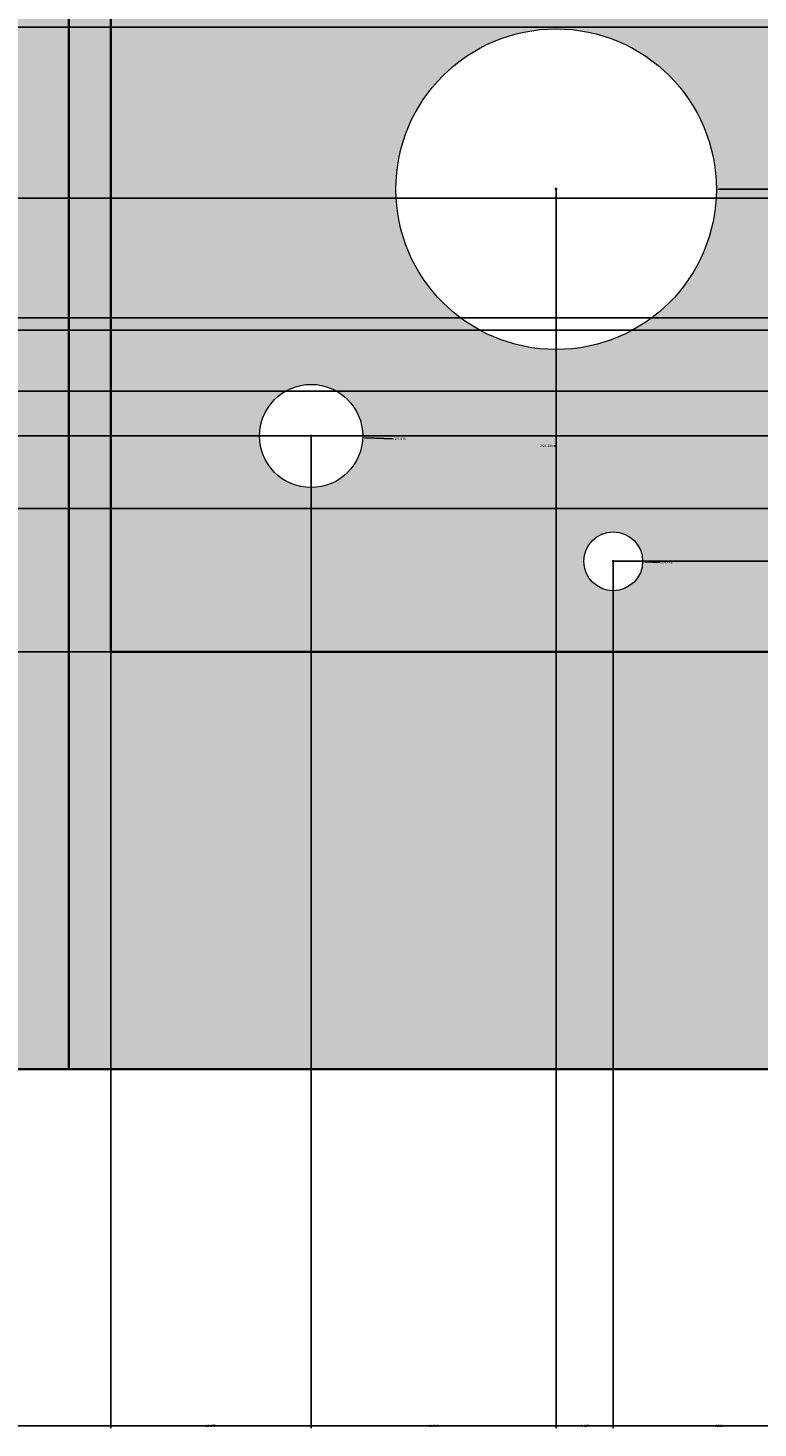
# Model space of a CAD drawing. Units: inches. Extents: x 73 to 607, y 92 to 651.
# Tile 7 of 18: x 448 to 504, y 116 to 222. Entities that reach past the tile are written whole.
import ezdxf

# ---------------------------------------------------------------- set-up
doc = ezdxf.new("R2010")
doc.units = ezdxf.units.IN
doc.header["$MEASUREMENT"] = 0
for name, color, linetype, lineweight in [('A-ANNO-DIMS', 2, 'Continuous', 18), ('A-ELEV', 7, 'Continuous', 35), ('A-ELEV-PANL', 7, 'Continuous', 18), ('A-ELEV-PATT-BKGD', 252, 'Continuous', 13), ('A-ELEV-PATT-SHAD', 8, 'Continuous', 13), ('A-ELEV-PATT-WALL', 254, 'Continuous', 13), ('A-ELEV-PATT-WOOD', 32, 'Continuous', 13)]:
    doc.layers.add(name, color=color, linetype=linetype, lineweight=lineweight)
doc.styles.get("Standard").update_dxf_attribs({"font": 'arial.ttf'})
doc.dimstyles.get("Standard").update_dxf_attribs({"dimtxt": 0.18, "dimasz": 0.18, "dimexe": 0.18, "dimexo": 0.0625, "dimgap": 0.09, "dimtad": 0, "dimtih": 1, "dimtoh": 1, "dimdec": 4, "dimzin": 0, "dimdsep": 46, "dimtxsty": 'Standard', "dimcen": 0.09, "dimadec": 0, "dimazin": 0, "dimtfac": 1, "dimtdec": 4, "dimtofl": 0, "dimtmove": 0, "dimatfit": 3, "dimfxl": 1, "dimtolj": 1, "dimtzin": 0, "dimarcsym": 0})

# ---------------------------------------------------------------- blocks, each defined once
blk = doc.blocks.new('*D4')
at = {"layer": 'A-ANNO-DIMS', "color": 0, "lineweight": -2, "transparency": 16777216}
for p, q in [((100.1, 143.14), (100.1, 116.02)), ((580.1, 143.14), (580.1, 116.02)), ((100.28, 116.2), (339.81, 116.2)), ((579.92, 116.2), (340.39, 116.2))]:
    blk.add_line(p, q, dxfattribs=at)
at = {"layer": 'A-ANNO-DIMS', "color": 0, "transparency": 16777216}
for points in [[(100.28, 116.23), (100.28, 116.17), (100.1, 116.2)], [(579.92, 116.23), (579.92, 116.17), (580.1, 116.2)]]:
    blk.add_solid(points, dxfattribs=at)
at = {"layer": 'Defpoints', "color": 0, "transparency": 16777216}
for p in [(100.1, 143.2), (580.1, 143.2), (580.1, 116.2)]:
    blk.add_point(p, dxfattribs=at)
at = {"layer": 'A-ANNO-DIMS', "color": 0, "transparency": 16777216, "insert": (340.1, 116.2), "char_height": 0.18, "attachment_point": 5}
blk.add_mtext('\\A1;480', dxfattribs=at)
blk = doc.blocks.new('*D15')
at = {"layer": 'A-ANNO-DIMS', "color": 0, "lineweight": -2, "transparency": 16777216}
for p, q in [((454.77, 174.8), (607.28, 174.8)), ((607.1, 174.62), (607.1, 159.19)), ((607.1, 143.38), (607.1, 158.82)), ((580.16, 143.2), (607.28, 143.2))]:
    blk.add_line(p, q, dxfattribs=at)
at = {"layer": 'A-ANNO-DIMS', "color": 0, "transparency": 16777216}
for points in [[(607.07, 174.62), (607.13, 174.62), (607.1, 174.8)], [(607.07, 143.38), (607.13, 143.38), (607.1, 143.2)]]:
    blk.add_solid(points, dxfattribs=at)
at = {"layer": 'Defpoints', "color": 0, "transparency": 16777216}
for p in [(454.7, 174.8), (607.1, 174.8), (580.1, 143.2)]:
    blk.add_point(p, dxfattribs=at)
at = {"layer": 'A-ANNO-DIMS', "color": 0, "transparency": 16777216, "insert": (607.1, 159), "char_height": 0.18, "attachment_point": 5}
blk.add_mtext('\\A1;31.6', dxfattribs=at)
blk = doc.blocks.new('*D16')
at = {"layer": 'A-ANNO-DIMS', "color": 0, "lineweight": -2, "transparency": 16777216}
for p, q in [((431.13, 185.66), (607.28, 185.66)), ((607.1, 185.48), (607.1, 180.41)), ((607.1, 174.98), (607.1, 180.05)), ((454.77, 174.8), (607.28, 174.8))]:
    blk.add_line(p, q, dxfattribs=at)
at = {"layer": 'A-ANNO-DIMS', "color": 0, "transparency": 16777216}
for points in [[(607.07, 185.48), (607.13, 185.48), (607.1, 185.66)], [(607.07, 174.98), (607.13, 174.98), (607.1, 174.8)]]:
    blk.add_solid(points, dxfattribs=at)
at = {"layer": 'Defpoints', "color": 0, "transparency": 16777216}
for p in [(431.07, 185.66), (607.1, 185.66), (454.7, 174.8)]:
    blk.add_point(p, dxfattribs=at)
at = {"layer": 'A-ANNO-DIMS', "color": 0, "transparency": 16777216, "insert": (607.1, 180.23), "char_height": 0.18, "attachment_point": 5}
blk.add_mtext('\\A1;10.86', dxfattribs=at)
blk = doc.blocks.new('*D17')
at = {"layer": 'A-ANNO-DIMS', "color": 0, "lineweight": -2, "transparency": 16777216}
for p, q in [((580.16, 262.3), (607.28, 262.3)), ((607.1, 262.12), (607.1, 224.16)), ((607.1, 185.84), (607.1, 223.8)), ((431.13, 185.66), (607.28, 185.66))]:
    blk.add_line(p, q, dxfattribs=at)
at = {"layer": 'A-ANNO-DIMS', "color": 0, "transparency": 16777216}
for points in [[(607.07, 262.12), (607.13, 262.12), (607.1, 262.3)], [(607.07, 185.84), (607.13, 185.84), (607.1, 185.66)]]:
    blk.add_solid(points, dxfattribs=at)
at = {"layer": 'Defpoints', "color": 0, "transparency": 16777216}
for p in [(580.1, 262.3), (607.1, 262.3), (431.07, 185.66)]:
    blk.add_point(p, dxfattribs=at)
at = {"layer": 'A-ANNO-DIMS', "color": 0, "transparency": 16777216, "insert": (607.1, 223.98), "char_height": 0.18, "attachment_point": 5}
blk.add_mtext('\\A1;76.64', dxfattribs=at)
blk = doc.blocks.new('*D40')
at = {"layer": 'A-ANNO-DIMS', "color": 0, "lineweight": -2, "transparency": 16777216}
for p, q in [((454.64, 256.63), (427.52, 256.63)), ((427.7, 256.45), (427.7, 215.9)), ((427.7, 174.98), (427.7, 215.54)), ((454.64, 174.8), (427.52, 174.8))]:
    blk.add_line(p, q, dxfattribs=at)
at = {"layer": 'A-ANNO-DIMS', "color": 0, "transparency": 16777216}
for points in [[(427.67, 256.45), (427.73, 256.45), (427.7, 256.63)], [(427.67, 174.98), (427.73, 174.98), (427.7, 174.8)]]:
    blk.add_solid(points, dxfattribs=at)
at = {"layer": 'Defpoints', "color": 0, "transparency": 16777216}
for p in [(427.7, 256.63), (454.7, 256.63), (454.7, 174.8)]:
    blk.add_point(p, dxfattribs=at)
at = {"layer": 'A-ANNO-DIMS', "color": 0, "transparency": 16777216, "insert": (427.7, 215.72), "char_height": 0.18, "attachment_point": 5}
blk.add_mtext('\\A1;81.83', dxfattribs=at)
blk = doc.blocks.new('*D62')
at = {"layer": 'A-ANNO-DIMS', "color": 0, "lineweight": -2, "transparency": 16777216}
for p, q in [((488.44, 209.74), (488.44, 209.92)), ((488.35, 209.83), (488.53, 209.83)), ((507.87, 209.83), (500.76, 209.83))]:
    blk.add_line(p, q, dxfattribs=at)
at = {"layer": 'A-ANNO-DIMS', "color": 0, "transparency": 16777216}
blk.add_solid([(500.76, 209.86), (500.76, 209.8), (500.58, 209.83)], dxfattribs=at)
at = {"layer": 'Defpoints', "color": 0, "transparency": 16777216}
for p in [(476.3, 209.83), (500.58, 209.83)]:
    blk.add_point(p, dxfattribs=at)
at = {"layer": 'A-ANNO-DIMS', "color": 0, "transparency": 16777216, "insert": (508.43, 209.83), "char_height": 0.18, "attachment_point": 5}
blk.add_mtext('\\A1;∅24.285', dxfattribs=at)
blk = doc.blocks.new('*D94')
at = {"layer": 'A-ANNO-DIMS', "color": 0, "lineweight": -2, "transparency": 16777216}
for p, q in [((377.02, 209.14), (607.28, 209.14)), ((607.1, 208.96), (607.1, 204.33)), ((607.1, 199.33), (607.1, 203.97)), ((363.32, 199.15), (607.28, 199.15))]:
    blk.add_line(p, q, dxfattribs=at)
at = {"layer": 'A-ANNO-DIMS', "color": 0, "transparency": 16777216}
for points in [[(607.07, 208.96), (607.13, 208.96), (607.1, 209.14)], [(607.07, 199.33), (607.13, 199.33), (607.1, 199.15)]]:
    blk.add_solid(points, dxfattribs=at)
at = {"layer": 'Defpoints', "color": 0, "transparency": 16777216}
for p in [(376.96, 209.14), (363.26, 199.15), (607.1, 199.15)]:
    blk.add_point(p, dxfattribs=at)
at = {"layer": 'A-ANNO-DIMS', "color": 0, "transparency": 16777216, "insert": (607.1, 204.15), "char_height": 0.18, "attachment_point": 5}
blk.add_mtext('\\A1;9.992', dxfattribs=at)
blk = doc.blocks.new('*D95')
at = {"layer": 'A-ANNO-DIMS', "color": 0, "lineweight": -2, "transparency": 16777216}
for p, q in [((363.87, 225.98), (607.28, 225.98)), ((607.1, 225.8), (607.1, 212.75)), ((607.1, 199.33), (607.1, 212.38)), ((363.32, 199.15), (607.28, 199.15))]:
    blk.add_line(p, q, dxfattribs=at)
at = {"layer": 'A-ANNO-DIMS', "color": 0, "transparency": 16777216}
for points in [[(607.07, 225.8), (607.13, 225.8), (607.1, 225.98)], [(607.07, 199.33), (607.13, 199.33), (607.1, 199.15)]]:
    blk.add_solid(points, dxfattribs=at)
at = {"layer": 'Defpoints', "color": 0, "transparency": 16777216}
for p in [(363.81, 225.98), (607.1, 225.98), (363.26, 199.15)]:
    blk.add_point(p, dxfattribs=at)
at = {"layer": 'A-ANNO-DIMS', "color": 0, "transparency": 16777216, "insert": (607.1, 212.57), "char_height": 0.18, "attachment_point": 5}
blk.add_mtext('\\A1;26.83', dxfattribs=at)
blk = doc.blocks.new('*D97')
at = {"layer": 'A-ANNO-DIMS', "color": 0, "lineweight": -2, "transparency": 16777216}
for p, q in [((387.58, 200.08), (607.28, 200.08)), ((607.1, 199.9), (607.1, 197.49)), ((607.1, 194.72), (607.1, 197.12)), ((396.75, 194.54), (607.28, 194.54))]:
    blk.add_line(p, q, dxfattribs=at)
at = {"layer": 'A-ANNO-DIMS', "color": 0, "transparency": 16777216}
for points in [[(607.07, 199.9), (607.13, 199.9), (607.1, 200.08)], [(607.07, 194.72), (607.13, 194.72), (607.1, 194.54)]]:
    blk.add_solid(points, dxfattribs=at)
at = {"layer": 'Defpoints', "color": 0, "transparency": 16777216}
for p in [(387.52, 200.08), (607.1, 200.08), (396.69, 194.54)]:
    blk.add_point(p, dxfattribs=at)
at = {"layer": 'A-ANNO-DIMS', "color": 0, "transparency": 16777216, "insert": (607.1, 197.31), "char_height": 0.18, "attachment_point": 5}
blk.add_mtext('\\A1;5.54', dxfattribs=at)
blk = doc.blocks.new('*D98')
at = {"layer": 'A-ANNO-DIMS', "color": 0, "lineweight": -2, "transparency": 16777216}
for p, q in [((377.02, 209.14), (607.28, 209.14)), ((607.1, 208.96), (607.1, 204.79)), ((607.1, 200.26), (607.1, 204.43)), ((387.58, 200.08), (607.28, 200.08))]:
    blk.add_line(p, q, dxfattribs=at)
at = {"layer": 'A-ANNO-DIMS', "color": 0, "transparency": 16777216}
for points in [[(607.07, 208.96), (607.13, 208.96), (607.1, 209.14)], [(607.07, 200.26), (607.13, 200.26), (607.1, 200.08)]]:
    blk.add_solid(points, dxfattribs=at)
at = {"layer": 'Defpoints', "color": 0, "transparency": 16777216}
for p in [(376.96, 209.14), (607.1, 209.14), (387.52, 200.08)]:
    blk.add_point(p, dxfattribs=at)
at = {"layer": 'A-ANNO-DIMS', "color": 0, "transparency": 16777216, "insert": (607.1, 204.61), "char_height": 0.18, "attachment_point": 5}
blk.add_mtext('\\A1;9.067', dxfattribs=at)
blk = doc.blocks.new('*D99')
at = {"layer": 'A-ANNO-DIMS', "color": 0, "lineweight": -2, "transparency": 16777216}
for p, q in [((373.32, 231.35), (607.28, 231.35)), ((607.1, 231.17), (607.1, 220.43)), ((607.1, 209.32), (607.1, 220.06)), ((377.02, 209.14), (607.28, 209.14))]:
    blk.add_line(p, q, dxfattribs=at)
at = {"layer": 'A-ANNO-DIMS', "color": 0, "transparency": 16777216}
for points in [[(607.07, 231.17), (607.13, 231.17), (607.1, 231.35)], [(607.07, 209.32), (607.13, 209.32), (607.1, 209.14)]]:
    blk.add_solid(points, dxfattribs=at)
at = {"layer": 'Defpoints', "color": 0, "transparency": 16777216}
for p in [(373.26, 231.35), (607.1, 231.35), (376.96, 209.14)]:
    blk.add_point(p, dxfattribs=at)
at = {"layer": 'A-ANNO-DIMS', "color": 0, "transparency": 16777216, "insert": (607.1, 220.25), "char_height": 0.18, "attachment_point": 5}
blk.add_mtext('\\A1;22.205', dxfattribs=at)
blk = doc.blocks.new('*D100')
at = {"layer": 'A-ANNO-DIMS', "color": 0, "lineweight": -2, "transparency": 16777216}
for p, q in [((382.95, 222.1), (607.28, 222.1)), ((607.1, 221.92), (607.1, 211.27)), ((607.1, 200.26), (607.1, 210.9)), ((387.58, 200.08), (607.28, 200.08))]:
    blk.add_line(p, q, dxfattribs=at)
at = {"layer": 'A-ANNO-DIMS', "color": 0, "transparency": 16777216}
for points in [[(607.07, 221.92), (607.13, 221.92), (607.1, 222.1)], [(607.07, 200.26), (607.13, 200.26), (607.1, 200.08)]]:
    blk.add_solid(points, dxfattribs=at)
at = {"layer": 'Defpoints', "color": 0, "transparency": 16777216}
for p in [(382.89, 222.1), (607.1, 222.1), (387.52, 200.08)]:
    blk.add_point(p, dxfattribs=at)
at = {"layer": 'A-ANNO-DIMS', "color": 0, "transparency": 16777216, "insert": (607.1, 211.09), "char_height": 0.18, "attachment_point": 5}
blk.add_mtext('\\A1;22.02', dxfattribs=at)
blk = doc.blocks.new('*D110')
at = {"layer": 'A-ANNO-DIMS', "color": 0, "lineweight": -2, "transparency": 16777216}
for p, q in [((469.88, 191.08), (469.88, 116.02)), ((454.7, 174.74), (454.7, 116.02)), ((454.88, 116.2), (461.84, 116.2)), ((469.7, 116.2), (462.75, 116.2))]:
    blk.add_line(p, q, dxfattribs=at)
at = {"layer": 'A-ANNO-DIMS', "color": 0, "transparency": 16777216}
for points in [[(454.88, 116.23), (454.88, 116.17), (454.7, 116.2)], [(469.7, 116.23), (469.7, 116.17), (469.88, 116.2)]]:
    blk.add_solid(points, dxfattribs=at)
at = {"layer": 'Defpoints', "color": 0, "transparency": 16777216}
for p in [(469.88, 191.14), (454.7, 174.8), (469.88, 116.2)]:
    blk.add_point(p, dxfattribs=at)
at = {"layer": 'A-ANNO-DIMS', "color": 0, "transparency": 16777216, "insert": (462.29, 116.2), "char_height": 0.18, "attachment_point": 5}
blk.add_mtext('\\A1;15.175', dxfattribs=at)
blk = doc.blocks.new('*D111')
at = {"layer": 'A-ANNO-DIMS', "color": 0, "lineweight": -2, "transparency": 16777216}
for p, q in [((488.44, 209.77), (488.44, 116.02)), ((469.88, 191.08), (469.88, 116.02)), ((470.06, 116.2), (478.71, 116.2)), ((488.26, 116.2), (479.62, 116.2))]:
    blk.add_line(p, q, dxfattribs=at)
at = {"layer": 'A-ANNO-DIMS', "color": 0, "transparency": 16777216}
for points in [[(470.06, 116.23), (470.06, 116.17), (469.88, 116.2)], [(488.26, 116.23), (488.26, 116.17), (488.44, 116.2)]]:
    blk.add_solid(points, dxfattribs=at)
at = {"layer": 'Defpoints', "color": 0, "transparency": 16777216}
for p in [(488.44, 209.83), (469.88, 191.14), (488.44, 116.2)]:
    blk.add_point(p, dxfattribs=at)
at = {"layer": 'A-ANNO-DIMS', "color": 0, "transparency": 16777216, "insert": (479.16, 116.2), "char_height": 0.18, "attachment_point": 5}
blk.add_mtext('\\A1;18.563', dxfattribs=at)
blk = doc.blocks.new('*D112')
at = {"layer": 'A-ANNO-DIMS', "color": 0, "lineweight": -2, "transparency": 16777216}
for p, q in [((488.44, 209.77), (488.44, 116.02)), ((492.77, 181.6), (492.77, 116.02)), ((488.62, 116.2), (490.21, 116.2)), ((492.59, 116.2), (491, 116.2))]:
    blk.add_line(p, q, dxfattribs=at)
at = {"layer": 'A-ANNO-DIMS', "color": 0, "transparency": 16777216}
for points in [[(488.62, 116.23), (488.62, 116.17), (488.44, 116.2)], [(492.59, 116.23), (492.59, 116.17), (492.77, 116.2)]]:
    blk.add_solid(points, dxfattribs=at)
at = {"layer": 'Defpoints', "color": 0, "transparency": 16777216}
for p in [(488.44, 209.83), (492.77, 181.66), (492.77, 116.2)]:
    blk.add_point(p, dxfattribs=at)
at = {"layer": 'A-ANNO-DIMS', "color": 0, "transparency": 16777216, "insert": (490.61, 116.2), "char_height": 0.18, "attachment_point": 5}
blk.add_mtext('\\A1;4.327', dxfattribs=at)
blk = doc.blocks.new('*D113')
at = {"layer": 'A-ANNO-DIMS', "color": 0, "lineweight": -2, "transparency": 16777216}
for p, q in [((508.96, 194.7), (508.96, 116.02)), ((492.77, 181.6), (492.77, 116.02)), ((492.95, 116.2), (500.48, 116.2)), ((508.78, 116.2), (501.25, 116.2))]:
    blk.add_line(p, q, dxfattribs=at)
at = {"layer": 'A-ANNO-DIMS', "color": 0, "transparency": 16777216}
for points in [[(492.95, 116.23), (492.95, 116.17), (492.77, 116.2)], [(508.78, 116.23), (508.78, 116.17), (508.96, 116.2)]]:
    blk.add_solid(points, dxfattribs=at)
at = {"layer": 'Defpoints', "color": 0, "transparency": 16777216}
for p in [(508.96, 194.77), (492.77, 181.66), (508.96, 116.2)]:
    blk.add_point(p, dxfattribs=at)
at = {"layer": 'A-ANNO-DIMS', "color": 0, "transparency": 16777216, "insert": (500.86, 116.2), "char_height": 0.18, "attachment_point": 5}
blk.add_mtext('\\A1;16.19', dxfattribs=at)
blk = doc.blocks.new('*D119')
at = {"layer": 'A-ANNO-DIMS', "color": 0, "lineweight": -2, "transparency": 16777216}
for p, q in [((469.82, 191.14), (72.92, 191.14)), ((73.1, 190.96), (73.1, 183.15)), ((73.1, 174.98), (73.1, 182.79)), ((454.64, 174.8), (72.92, 174.8))]:
    blk.add_line(p, q, dxfattribs=at)
at = {"layer": 'A-ANNO-DIMS', "color": 0, "transparency": 16777216}
for points in [[(73.07, 190.96), (73.13, 190.96), (73.1, 191.14)], [(73.07, 174.98), (73.13, 174.98), (73.1, 174.8)]]:
    blk.add_solid(points, dxfattribs=at)
at = {"layer": 'Defpoints', "color": 0, "transparency": 16777216}
for p in [(73.1, 191.14), (469.88, 191.14), (454.7, 174.8)]:
    blk.add_point(p, dxfattribs=at)
at = {"layer": 'A-ANNO-DIMS', "color": 0, "transparency": 16777216, "insert": (73.1, 182.97), "char_height": 0.18, "attachment_point": 5}
blk.add_mtext('\\A1;16.34', dxfattribs=at)
blk = doc.blocks.new('*D120')
at = {"layer": 'A-ANNO-DIMS', "color": 0, "lineweight": -2, "transparency": 16777216}
for p, q in [((468.55, 225.73), (607.28, 225.73)), ((607.1, 225.55), (607.1, 208.62)), ((607.1, 191.32), (607.1, 208.25)), ((469.94, 191.14), (607.28, 191.14))]:
    blk.add_line(p, q, dxfattribs=at)
at = {"layer": 'A-ANNO-DIMS', "color": 0, "transparency": 16777216}
for points in [[(607.07, 225.55), (607.13, 225.55), (607.1, 225.73)], [(607.07, 191.32), (607.13, 191.32), (607.1, 191.14)]]:
    blk.add_solid(points, dxfattribs=at)
at = {"layer": 'Defpoints', "color": 0, "transparency": 16777216}
for p in [(468.48, 225.73), (607.1, 225.73), (469.88, 191.14)]:
    blk.add_point(p, dxfattribs=at)
at = {"layer": 'A-ANNO-DIMS', "color": 0, "transparency": 16777216, "insert": (607.1, 208.43), "char_height": 0.18, "attachment_point": 5}
blk.add_mtext('\\A1;34.585', dxfattribs=at)
blk = doc.blocks.new('*D122')
at = {"layer": 'A-ANNO-DIMS', "color": 0, "lineweight": -2, "transparency": 16777216}
for p, q in [((509.02, 194.77), (607.28, 194.77)), ((607.1, 194.59), (607.1, 188.39)), ((607.1, 181.84), (607.1, 188.03)), ((492.83, 181.66), (607.28, 181.66))]:
    blk.add_line(p, q, dxfattribs=at)
at = {"layer": 'A-ANNO-DIMS', "color": 0, "transparency": 16777216}
for points in [[(607.07, 194.59), (607.13, 194.59), (607.1, 194.77)], [(607.07, 181.84), (607.13, 181.84), (607.1, 181.66)]]:
    blk.add_solid(points, dxfattribs=at)
at = {"layer": 'Defpoints', "color": 0, "transparency": 16777216}
for p in [(508.96, 194.77), (492.77, 181.66), (607.1, 181.66)]:
    blk.add_point(p, dxfattribs=at)
at = {"layer": 'A-ANNO-DIMS', "color": 0, "transparency": 16777216, "insert": (607.1, 188.21), "char_height": 0.18, "attachment_point": 5}
blk.add_mtext('\\A1;13.11', dxfattribs=at)
blk = doc.blocks.new('*D161')
at = {"layer": 'A-ANNO-DIMS', "color": 0, "lineweight": -2, "transparency": 16777216}
for p, q in [((488.44, 209.74), (488.44, 209.92)), ((488.35, 209.83), (488.53, 209.83)), ((488.44, 190.4), (488.44, 197.51)), ((488.26, 190.4), (488.44, 190.4))]:
    blk.add_line(p, q, dxfattribs=at)
at = {"layer": 'A-ANNO-DIMS', "color": 0, "transparency": 16777216}
blk.add_solid([(488.41, 197.51), (488.47, 197.51), (488.44, 197.69)], dxfattribs=at)
at = {"layer": 'Defpoints', "color": 0, "transparency": 16777216}
for p in [(488.44, 221.97), (488.44, 197.69)]:
    blk.add_point(p, dxfattribs=at)
at = {"layer": 'A-ANNO-DIMS', "color": 0, "transparency": 16777216, "insert": (487.7, 190.4), "char_height": 0.18, "attachment_point": 5}
blk.add_mtext('\\A1;∅24.285', dxfattribs=at)
blk = doc.blocks.new('*D165')
at = {"layer": 'A-ANNO-DIMS', "color": 0, "lineweight": -2, "transparency": 16777216}
for p, q in [((469.79, 191.14), (469.97, 191.14)), ((469.88, 191.05), (469.88, 191.23)), ((476.13, 190.92), (473.96, 190.99))]:
    blk.add_line(p, q, dxfattribs=at)
at = {"layer": 'A-ANNO-DIMS', "color": 0, "transparency": 16777216}
blk.add_solid([(473.97, 191.02), (473.96, 190.96), (473.78, 191)], dxfattribs=at)
at = {"layer": 'Defpoints', "color": 0, "transparency": 16777216}
for p in [(465.97, 191.28), (473.78, 191)]:
    blk.add_point(p, dxfattribs=at)
at = {"layer": 'A-ANNO-DIMS', "color": 0, "transparency": 16777216, "insert": (476.62, 190.92), "char_height": 0.18, "attachment_point": 5}
blk.add_mtext('\\A1;∅7.816', dxfattribs=at)
blk = doc.blocks.new('*D168')
at = {"layer": 'A-ANNO-DIMS', "color": 0, "lineweight": -2, "transparency": 16777216}
for p, q in [((492.68, 181.66), (492.86, 181.66)), ((492.77, 181.57), (492.77, 181.75)), ((496.34, 181.57), (495.18, 181.6))]:
    blk.add_line(p, q, dxfattribs=at)
at = {"layer": 'A-ANNO-DIMS', "color": 0, "transparency": 16777216}
blk.add_solid([(495.18, 181.63), (495.18, 181.57), (495, 181.6)], dxfattribs=at)
at = {"layer": 'Defpoints', "color": 0, "transparency": 16777216}
for p in [(490.54, 181.72), (495, 181.6)]:
    blk.add_point(p, dxfattribs=at)
at = {"layer": 'A-ANNO-DIMS', "color": 0, "transparency": 16777216, "insert": (496.83, 181.57), "char_height": 0.18, "attachment_point": 5}
blk.add_mtext('\\A1;∅4.463', dxfattribs=at)

msp = doc.modelspace()

# ---------------------------------------------------------------- hatches: boundary and pattern name
at = {"layer": 'A-ELEV-PATT-BKGD'}
h = msp.add_hatch(color=256, dxfattribs=at)
h.dxf.hatch_style = 1
h.paths.add_polyline_path([(321.3008, 479.2042), (312.3008, 479.2042), (312.3008, 478.7576), (312.3008, 412.636), (321.3008, 412.636)])
h.paths.add_polyline_path([(312.3008, 504.7576), (256.4726, 504.7576), (256.4726, 503.4576), (312.3008, 503.4576)], flags=17)
h.paths.add_polyline_path([(321.3008, 543.1576), (321.3008, 552.1576), (320.3257, 552.1576), (312.3008, 552.1576), (256.4726, 552.1576), (256.4726, 543.1576), (312.3008, 543.1576), (312.3008, 479.2042), (321.3008, 479.2042)])
h.paths.add_polyline_path([(451.5214, 412.636), (256.4726, 412.636), (256.4726, 403.636), (442.5214, 403.636), (442.5214, 320.2042), (206.1343, 320.2042), (206.1343, 320.9135), (206.1343, 403.636), (256.4726, 403.636), (256.4726, 412.636), (201.6343, 412.636), (201.6343, 320.9135), (201.6343, 320.2042), (201.6343, 311.2042), (256.4726, 311.2042), (451.5214, 311.2042)])
h.paths.add_polyline_path([(431.07, 258.6914), (369.5339, 258.6914), (369.5339, 247.4054), (396.692, 247.4054), (425.07, 247.4054), (425.07, 194.7312), (396.692, 194.6197), (396.692, 194.5366), (369.5339, 194.5366), (369.5339, 185.6619), (431.07, 185.6619)])
h.paths.add_polyline_path([(580.0983, 262.3024), (451.5214, 262.3024), (451.5214, 143.2042), (580.0983, 143.2042)])
h.paths.add_polyline_path([(454.7049, 174.802), (454.7049, 256.6321), (577.9249, 256.6321), (577.9249, 174.802)], flags=16)
h.paths.add_polyline_path([(465.9716, 191.1416, -1), (473.7874, 191.1416, -1)], flags=0)
h.paths.add_polyline_path([(490.5373, 181.6586, -1), (494.9999, 181.6586, -1)], flags=0)
h.paths.add_polyline_path([(476.2996, 209.8287, -1), (500.5844, 209.8287, -1)], flags=0)
h.paths.add_polyline_path([(505.3326, 194.7675, -1), (512.5843, 194.7675, -1)], flags=0)
h.paths.add_polyline_path([(520.9613, 186.679, -1), (526.544, 186.679, -1)], flags=0)
h.paths.add_polyline_path([(466.8103, 225.7267, -1), (470.1573, 225.7267, -1)], flags=0)
h.paths.add_polyline_path([(527.1059, 203.6926, -1), (536.0311, 203.6926, -1)], flags=0)
h.paths.add_polyline_path([(504.775, 232.6995, -1), (513.7002, 232.6995, -1)], flags=0)
h.paths.add_polyline_path([(546.9241, 183.611, -1), (554.7336, 183.611, -1)], flags=0)
h.paths.add_polyline_path([(459.5544, 243.856, -1), (466.8061, 243.856, -1)], flags=0)
h.paths.add_polyline_path([(476.3045, 246.924, -1), (488.5767, 246.924, -1)], flags=0)
h.paths.add_polyline_path([(529.9044, 226.8424, -1), (556.68, 226.8424, -1)], flags=0)
h.paths.add_polyline_path([(554.1814, 203.9716, -1), (561.4331, 203.9716, -1)], flags=0)
h.paths.add_polyline_path([(567.8561, 193.3729, -1), (570.6475, 193.3729, -1)], flags=0)
h.paths.add_polyline_path([(522.3584, 250.271, -1), (525.7053, 250.271, -1)], flags=0)
h.paths.add_polyline_path([(561.9965, 245.2506, -1), (567.5748, 245.2506, -1)], flags=0)
h.paths.add_polyline_path([(347.8686, 194.5366), (341.8686, 194.5366), (341.8686, 194.5452), (314.0144, 194.5452), (314.0144, 188.5452), (347.8686, 188.5452)])
h.paths.add_polyline_path([(347.8686, 253.4054), (314.0144, 253.4054), (314.0144, 247.4054), (341.8686, 247.4054), (347.8686, 247.4054)])
h.paths.add_polyline_path([(304.3559, 253.4054), (298.3559, 253.4054), (298.3559, 188.5452), (304.3559, 188.5452)])
h.paths.add_polyline_path([(450.6603, 552.1576), (369.9727, 552.1576), (369.9727, 479.2042), (374.4727, 479.2042), (374.4727, 547.6576), (446.1603, 547.6576), (446.1603, 479.2042), (450.6603, 479.2042)])
h.paths.add_polyline_path([(374.4727, 479.2042), (369.9727, 479.2042), (369.9727, 465.0632), (374.4727, 465.0632)])
h.paths.add_polyline_path([(450.6603, 479.2042), (446.1603, 479.2042), (446.1603, 465.0632), (450.6603, 465.0632)])
h.paths.add_polyline_path([(256.4726, 281.6039), (109.0983, 281.6039), (100.0983, 281.6039), (100.0983, 167.2042), (100.0983, 143.2042), (109.0983, 143.2042), (109.0983, 167.2042), (109.0983, 272.6039), (256.4726, 272.6039)])
at = {"layer": 'A-ELEV-PATT-SHAD'}
h = msp.add_hatch(color=256, dxfattribs=at)
h.dxf.hatch_style = 1
h.paths.add_polyline_path([(451.5214, 412.636), (256.4726, 412.636), (256.4726, 403.636), (442.5214, 403.636), (442.5214, 320.2042), (206.1343, 320.2042), (206.1343, 320.9135), (206.1343, 403.636), (256.4726, 403.636), (256.4726, 412.636), (201.6343, 412.636), (201.6343, 320.9135), (201.6343, 320.2042), (201.6343, 311.2042), (256.4726, 311.2042), (451.5214, 311.2042)])
h.paths.add_polyline_path([(580.0983, 262.3024), (451.5214, 262.3024), (451.5214, 143.2042), (580.0983, 143.2042)])
h.paths.add_polyline_path([(454.7049, 174.802), (454.7049, 256.6321), (577.9249, 256.6321), (577.9249, 174.802)], flags=16)
h.paths.add_polyline_path([(465.9716, 191.1416, -1), (473.7874, 191.1416, -1)], flags=0)
h.paths.add_polyline_path([(490.5373, 181.6586, -1), (494.9999, 181.6586, -1)], flags=0)
h.paths.add_polyline_path([(476.2996, 209.8287, -1), (500.5844, 209.8287, -1)], flags=0)
h.paths.add_polyline_path([(505.3326, 194.7675, -1), (512.5843, 194.7675, -1)], flags=0)
h.paths.add_polyline_path([(520.9613, 186.679, -1), (526.544, 186.679, -1)], flags=0)
h.paths.add_polyline_path([(466.8103, 225.7267, -1), (470.1573, 225.7267, -1)], flags=0)
h.paths.add_polyline_path([(527.1059, 203.6926, -1), (536.0311, 203.6926, -1)], flags=0)
h.paths.add_polyline_path([(459.5544, 243.856, -1), (466.8061, 243.856, -1)], flags=0)
h.paths.add_polyline_path([(504.775, 232.6995, -1), (513.7002, 232.6995, -1)], flags=0)
h.paths.add_polyline_path([(476.3045, 246.924, -1), (488.5767, 246.924, -1)], flags=0)
h.paths.add_polyline_path([(546.9241, 183.611, -1), (554.7336, 183.611, -1)], flags=0)
h.paths.add_polyline_path([(529.9044, 226.8424, -1), (556.68, 226.8424, -1)], flags=0)
h.paths.add_polyline_path([(554.1814, 203.9716, -1), (561.4331, 203.9716, -1)], flags=0)
h.paths.add_polyline_path([(522.3584, 250.271, -1), (525.7053, 250.271, -1)], flags=0)
h.paths.add_polyline_path([(567.8561, 193.3729, -1), (570.6475, 193.3729, -1)], flags=0)
h.paths.add_polyline_path([(561.9965, 245.2506, -1), (567.5748, 245.2506, -1)], flags=0)
h.paths.add_polyline_path([(431.07, 258.6914), (369.5339, 258.6914), (369.5339, 247.4054), (396.692, 247.4054), (425.07, 247.4054), (425.07, 194.7312), (396.692, 194.6197), (396.692, 194.5366), (369.5339, 194.5366), (369.5339, 185.6619), (431.07, 185.6619)])
h.paths.add_polyline_path([(347.8686, 253.4054), (314.0144, 253.4054), (314.0144, 247.4054), (341.8686, 247.4054), (347.8686, 247.4054)])
h.paths.add_polyline_path([(304.3559, 253.4054), (298.3559, 253.4054), (298.3559, 188.5452), (304.3559, 188.5452)])
h.paths.add_polyline_path([(347.8686, 194.5366), (341.8686, 194.5366), (341.8686, 194.5452), (314.0144, 194.5452), (314.0144, 188.5452), (347.8686, 188.5452)])
at = {"layer": 'A-ELEV-PATT-WALL'}
h = msp.add_hatch(color=256, dxfattribs=at)
h.dxf.hatch_style = 1
h.paths.add_polyline_path([(509.9692, 483.857), (450.6603, 483.857), (450.6603, 465.0632), (446.1603, 465.0632), (446.1603, 484.2142), (374.4727, 484.2142), (374.4727, 465.0632), (369.9727, 465.0632), (369.9727, 484.2142), (321.3008, 484.2142), (321.3008, 412.636), (451.5214, 412.636), (451.5214, 311.2042), (314.0144, 311.2042), (314.0144, 253.4054), (347.8686, 253.4054), (347.8686, 247.4054), (369.5339, 247.4054), (369.5339, 258.6914), (431.07, 258.6914), (431.07, 185.6619), (369.5339, 185.6619), (369.5339, 194.5366), (347.8686, 194.5366), (347.8686, 188.5452), (314.0144, 188.5452), (314.0144, 143.2042), (451.5214, 143.2042), (451.5214, 262.3024), (580.0983, 262.3024), (580.0983, 311.2042), (509.9692, 311.2042)])
h.paths.add_polyline_path([(304.3559, 311.2042), (256.4726, 311.2042), (256.4726, 167.2042), (256.4726, 143.2042), (304.3559, 143.2042), (304.3559, 188.5452), (298.3559, 188.5452), (298.3559, 253.4054), (304.3559, 253.4054)])
at = {"layer": 'A-ELEV-PATT-WOOD'}
h = msp.add_hatch(color=256, dxfattribs=at)
h.dxf.hatch_style = 1
h.paths.add_polyline_path([(577.9249, 256.6321), (454.7049, 256.6321), (454.7049, 174.802), (577.9249, 174.802)])
h.paths.add_polyline_path([(476.2996, 209.8287, -1), (500.5844, 209.8287, -1)], flags=16)
h.paths.add_polyline_path([(473.7874, 191.1416, -1), (465.9716, 191.1416, -1)], flags=16)
h.paths.add_polyline_path([(466.8103, 225.7267, -1), (470.1573, 225.7267, -1)], flags=16)
h.paths.add_polyline_path([(459.5544, 243.856, -1), (466.8061, 243.856, -1)], flags=16)
h.paths.add_polyline_path([(494.9999, 181.6586, -1), (490.5373, 181.6586, -1)], flags=16)
h.paths.add_polyline_path([(476.3045, 246.924, -1), (488.5767, 246.924, -1)], flags=16)
h.paths.add_polyline_path([(512.5843, 194.7675, -1), (505.3326, 194.7675, -1)], flags=16)
h.paths.add_polyline_path([(504.775, 232.6995, -1), (513.7002, 232.6995, -1)], flags=16)
h.paths.add_polyline_path([(526.544, 186.679, -1), (520.9613, 186.679, -1)], flags=16)
h.paths.add_polyline_path([(536.0311, 203.6926, -1), (527.1059, 203.6926, -1)], flags=16)
h.paths.add_polyline_path([(529.9044, 226.8424, -1), (556.68, 226.8424, -1)], flags=16)
h.paths.add_polyline_path([(522.3584, 250.271, -1), (525.7053, 250.271, -1)], flags=16)
h.paths.add_polyline_path([(554.7336, 183.611, -1), (546.9241, 183.611, -1)], flags=16)
h.paths.add_polyline_path([(561.4331, 203.9716, -1), (554.1814, 203.9716, -1)], flags=16)
h.paths.add_polyline_path([(561.9965, 245.2506, -1), (567.5748, 245.2506, -1)], flags=16)
h.paths.add_polyline_path([(570.6475, 193.3729, -1), (567.8561, 193.3729, -1)], flags=16)

# ---------------------------------------------------------------- linework, layer by layer
at = {"layer": 'A-ELEV'}
msp.add_line((100.0983, 143.2042), (580.0983, 143.2042), dxfattribs=at)
for points in [[(580.0983, 143.2042), (451.5214, 143.2042), (451.5214, 262.3024), (580.0983, 262.3024)], [(454.7049, 256.6321), (577.9249, 256.6321), (577.9249, 174.802), (454.7049, 174.802)]]:
    msp.add_lwpolyline(points, close=True, dxfattribs=at)
at = {"layer": 'A-ELEV-PANL'}
for centre, radius in [((488.442, 209.8287), 12.1424), ((469.8795, 191.1416), 3.9079), ((492.7686, 181.6586), 2.2313)]:
    msp.add_circle(centre, radius, dxfattribs=at)

# ---------------------------------------------------------------- dimensions: what is measured, and where the dimension line sits
at = {"layer": 'A-ANNO-DIMS'}
for base, p1, p2, override, picture, middle in [((607.0983, 262.3024), (431.07, 185.6619), (580.0983, 262.3024), {"dimdec": 2, "dimlfac": 1, "dimrnd": 0, "dimzin": 0, "dimdsep": 46, "dimlunit": 2}, '*D17', (607.0983, 223.9821)), ((427.7049, 256.6321), (454.7049, 174.802), (454.7049, 256.6321), {"dimdec": 2, "dimlfac": 1, "dimrnd": 0, "dimzin": 0, "dimdsep": 46, "dimlunit": 2}, '*D40', (427.7049, 215.7171)), ((607.0983, 231.3482), (376.9603, 209.1433), (373.2566, 231.3482), {"dimdec": 3, "dimlfac": 1, "dimrnd": 0, "dimzin": 0, "dimdsep": 46, "dimlunit": 2}, '*D99', (607.0983, 220.2458)), ((607.0983, 225.982), (363.2564, 199.1512), (363.8119, 225.982), {"dimdec": 2, "dimlfac": 1, "dimrnd": 0, "dimzin": 0, "dimdsep": 46, "dimlunit": 2}, '*D95', (607.0983, 212.5666)), ((607.0983, 225.7267), (469.8795, 191.1416), (468.4838, 225.7267), {"dimdec": 3, "dimlfac": 1, "dimrnd": 0, "dimzin": 0, "dimdsep": 46, "dimlunit": 2}, '*D120', (607.0983, 208.4342)), ((607.0983, 222.0962), (387.5161, 200.0764), (382.8864, 222.0962), {"dimdec": 2, "dimlfac": 1, "dimrnd": 0, "dimzin": 0, "dimdsep": 46, "dimlunit": 2}, '*D100', (607.0983, 211.0863)), ((607.0983, 199.1512), (376.9603, 209.1433), (363.2564, 199.1512), {"dimdec": 3, "dimlfac": 1, "dimrnd": 0, "dimzin": 0, "dimdsep": 46, "dimlunit": 2}, '*D94', (607.0983, 204.1472)), ((607.0983, 209.1433), (387.5161, 200.0764), (376.9603, 209.1433), {"dimdec": 3, "dimlfac": 1, "dimrnd": 0, "dimzin": 0, "dimdsep": 46, "dimlunit": 2}, '*D98', (607.0983, 204.6098)), ((607.0983, 200.0764), (396.692, 194.5366), (387.5161, 200.0764), {"dimdec": 2, "dimlfac": 1, "dimrnd": 0, "dimzin": 0, "dimdsep": 46, "dimlunit": 2}, '*D97', (607.0983, 197.3065)), ((607.0983, 181.6586), (508.9585, 194.7675), (492.7686, 181.6586), {"dimdec": 2, "dimlfac": 1, "dimrnd": 0, "dimzin": 0, "dimdsep": 46, "dimlunit": 2}, '*D122', (607.0983, 188.213)), ((73.0983, 191.1416), (454.7049, 174.802), (469.8795, 191.1416), {"dimdec": 2, "dimlfac": 1, "dimrnd": 0, "dimzin": 0, "dimdsep": 46, "dimlunit": 2}, '*D119', (73.0983, 182.9718)), ((607.0983, 185.6619), (454.7049, 174.802), (431.07, 185.6619), {"dimdec": 2, "dimlfac": 1, "dimrnd": 0, "dimzin": 0, "dimdsep": 46, "dimlunit": 2}, '*D16', (607.0983, 180.232)), ((607.0983, 174.802), (580.0983, 143.2042), (454.7049, 174.802), {"dimdec": 1, "dimlfac": 1, "dimrnd": 0, "dimzin": 0, "dimdsep": 46, "dimlunit": 2}, '*D15', (607.0983, 159.0031))]:
    dim = msp.add_linear_dim(base=base, p1=p1, p2=p2, angle=90, dimstyle='Standard', override=override, dxfattribs=at)
    dim.commit()
    dim.dimension.update_dxf_attribs({"geometry": picture, "text_midpoint": middle})
for p1, p2, picture, middle in [((488.444, 221.9711), (488.44, 197.6863), '*D161', (487.6966, 190.4009)), ((476.2996, 209.8284), (500.5844, 209.829), '*D62', (507.8699, 209.8292)), ((465.9741, 191.2826), (473.7848, 191.0005), '*D165', (476.128, 190.9159)), ((490.5381, 181.7164), (494.9992, 181.6008), '*D168', (496.3375, 181.5661))]:
    dim = msp.add_diameter_dim_2p(p1=p1, p2=p2, dimstyle='Standard', override={"dimdec": 3, "dimlfac": 1, "dimrnd": 0, "dimzin": 0, "dimdsep": 46, "dimlunit": 2}, dxfattribs=at)
    dim.commit()
    dim.dimension.update_dxf_attribs({"geometry": picture, "text_midpoint": middle, "dimtype": 163})
for base, p1, p2, override, picture, middle in [((488.44201, 116.2042), (469.87948, 191.1416), (488.44201, 209.82871), {"dimdec": 3, "dimlfac": 1, "dimrnd": 0, "dimzin": 0, "dimdsep": 46, "dimlunit": 2}, '*D111', (479.16074, 116.2042)), ((492.7686, 116.2042), (488.442, 209.8287), (492.7686, 181.6586), {"dimdec": 3, "dimlfac": 1, "dimrnd": 0, "dimzin": 0, "dimdsep": 46, "dimlunit": 2}, '*D112', (490.6053, 116.2042)), ((508.9585, 116.2042), (492.7686, 181.6586), (508.9585, 194.7675), {"dimdec": 2, "dimlfac": 1, "dimrnd": 0, "dimzin": 0, "dimdsep": 46, "dimlunit": 2}, '*D113', (500.8636, 116.2042)), ((469.8795, 116.2042), (454.7049, 174.802), (469.8795, 191.1416), {"dimdec": 3, "dimlfac": 1, "dimrnd": 0, "dimzin": 0, "dimdsep": 46, "dimlunit": 2}, '*D110', (462.2922, 116.2042)), ((580.0983, 116.2042), (100.0983, 143.2042), (580.0983, 143.2042), {"dimdec": 0, "dimlfac": 1, "dimrnd": 0, "dimzin": 0, "dimdsep": 46, "dimlunit": 2}, '*D4', (340.0983, 116.2042))]:
    dim = msp.add_linear_dim(base=base, p1=p1, p2=p2, dimstyle='Standard', override=override, dxfattribs=at)
    dim.commit()
    dim.dimension.update_dxf_attribs({"geometry": picture, "text_midpoint": middle})

doc.saveas('drawing.dxf')
